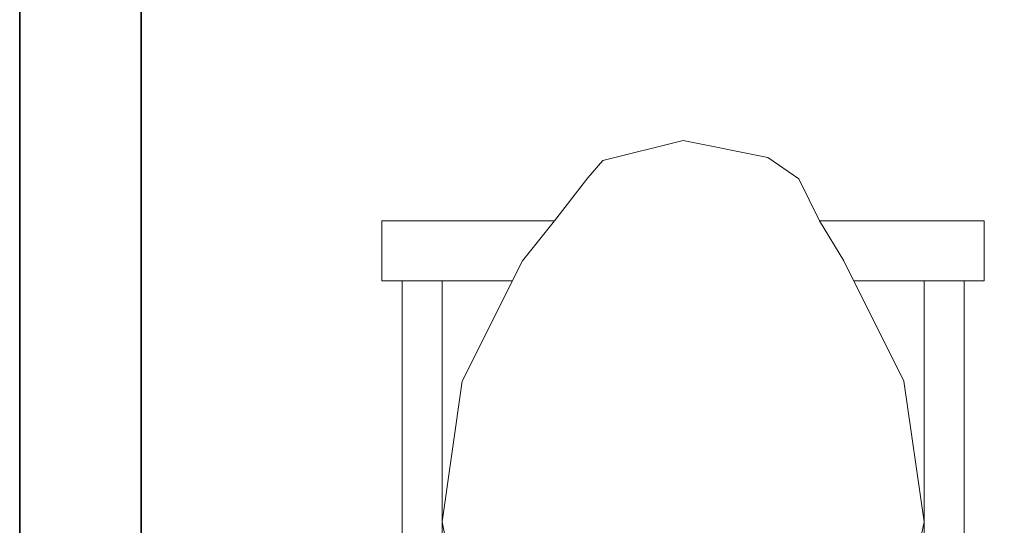
# Model space of a CAD drawing. Units: inches. Extents: x 64 to 1167, y 117 to 939.
# Tile 34 of 56: x 1040 to 1072, y 460 to 476. Entities that reach past the tile are written whole.
import ezdxf

# ---------------------------------------------------------------- set-up
doc = ezdxf.new("R2010")
doc.units = ezdxf.units.IN
doc.header["$MEASUREMENT"] = 0
doc.layers.add('A-FLOR-FIXT', color=8, linetype='Continuous', lineweight=18)
doc.layers.add('A-SECT', color=7, linetype='Continuous', lineweight=35)

# ---------------------------------------------------------------- blocks, each defined once
blk = doc.blocks.new('A$C02040E19')
for p, q in [((201.6, 890.4, 10), (268.8, 907.2, 10)), ((268.8, 907.2, 10), (339.63, 893.03, 10)), ((189.02, 876, 10), (201.6, 890.4, 10)), ((339.63, 893.03, 10), (365.72, 875.01, 10)), ((161.28, 840, 10), (189.02, 876, 10)), ((365.72, 875.01, 10), (383.04, 840, 10)), ((16.8, 840, 10), (161.28, 840, 10)), ((16.8, 840, 10), (16.8, 789.6, 10)), ((16.8, 789.6, 10), (16.8, 840, 10)), ((134.4, 806.4, 10), (161.28, 840, 10)), ((383.04, 840, 10), (520.8, 840, 10)), ((383.04, 840, 10), (403.2, 806.4, 10)), ((520.8, 840, 10), (520.8, 789.6, 10)), ((520.8, 840, 10), (520.8, 789.6, 10)), ((84, 705.6, 10), (134.4, 806.4, 10)), ((403.2, 806.4, 10), (453.6, 705.6, 10)), ((33.6, 789.6, 10), (16.8, 789.6, 10)), ((126, 789.6, 10), (33.6, 789.6, 10)), ((33.6, 403.2, 10), (33.6, 789.6, 10)), ((33.6, 403.2, 10), (33.6, 789.6, 10)), ((67.2, 789.6, 10), (67.2, 403.2, 10)), ((504, 789.6, 10), (411.6, 789.6, 10)), ((470.4, 789.6, 10), (470.4, 403.2, 10)), ((504, 789.6, 10), (504, 403.2, 10)), ((504, 789.6, 10), (504, 403.2, 10)), ((520.8, 789.6, 10), (504, 789.6, 10)), ((84, 705.6, 10), (67.2, 588, 10)), ((453.6, 705.6, 10), (470.4, 588, 10)), ((84, 504, 10), (67.2, 588, 10)), ((84, 504, 10), (67.2, 588, 10)), ((470.4, 588, 10), (453.6, 504, 10)), ((470.4, 588, 10), (453.6, 504, 10)), ((134.4, 436.8, 10), (84, 504, 10)), ((134.4, 436.8, 10), (84, 504, 10)), ((453.6, 504, 10), (403.2, 436.8, 10)), ((403.2, 436.8, 10), (453.6, 504, 10)), ((184.8, 420, 10), (134.4, 436.8, 10)), ((134.4, 436.8, 10), (184.8, 420, 10)), ((403.2, 436.8, 10), (352.8, 420, 10)), ((403.2, 436.8, 10), (352.8, 420, 10)), ((117.6, 403.2, 10), (134.4, 420, 10)), ((134.4, 420, 10), (117.6, 403.2, 10)), ((151.2, 420, 10), (134.4, 420, 10)), ((151.2, 420, 10), (134.4, 420, 10)), ((151.2, 420, 10), (168, 420, 10)), ((168, 420, 10), (151.2, 420, 10)), ((201.6, 420, 10), (168, 420, 10)), ((201.6, 420, 10), (168, 420, 10)), ((201.6, 420, 10), (235.2, 420, 10)), ((201.6, 420, 10), (235.2, 420, 10)), ((268.8, 420, 10), (235.2, 420, 10)), ((268.8, 420, 10), (235.2, 420, 10)), ((268.8, 420, 10), (319.2, 420, 10)), ((268.8, 420, 10), (319.2, 420, 10)), ((336, 420, 10), (319.2, 420, 10)), ((336, 420, 10), (319.2, 420, 10)), ((336, 420, 10), (369.6, 420, 10)), ((369.6, 420, 10), (336, 420, 10)), ((386.4, 420, 10), (369.6, 420, 10)), ((386.4, 420, 10), (369.6, 420, 10)), ((386.4, 420, 10), (403.2, 420, 10)), ((403.2, 420, 10), (386.4, 420, 10)), ((403.2, 420, 10), (420, 403.2, 10)), ((420, 403.2, 10), (403.2, 420, 10)), ((0, 403.2, 10), (0, 285.6, 10)), ((0, 403.2, 10), (33.6, 403.2, 10)), ((33.6, 403.2, 10), (504, 403.2, 10)), ((504, 403.2, 10), (537.6, 403.2, 10)), ((537.6, 403.2, 10), (537.6, 285.6, 10)), ((84, 218.4, 10), (0, 285.6, 10)), ((537.6, 285.6, 10), (453.6, 218.4, 10)), ((100.8, 218.4, 10), (84, 218.4, 10)), ((168, 151.2, 10), (100.8, 218.4, 10)), ((100.8, 218.4, 10), (436.8, 218.4, 10)), ((436.8, 218.4, 10), (369.6, 151.2, 10)), ((436.8, 218.4, 10), (453.6, 218.4, 10)), ((151.2, 16.8, 10), (168, 151.2, 10)), ((168, 151.2, 10), (369.6, 151.2, 10)), ((369.6, 151.2, 10), (386.4, 16.8, 10)), ((151.2, 16.8, 10), (117.6, 16.8, 10)), ((117.6, 0, 10), (117.6, 16.8, 10)), ((151.2, 16.8, 10), (386.4, 16.8, 10)), ((386.4, 16.8, 10), (420, 16.8, 10)), ((420, 16.8, 10), (420, 0, 10)), ((117.6, 0, 10), (420, 0, 10))]:
    blk.add_line(p, q)

msp = doc.modelspace()

# ---------------------------------------------------------------- linework, layer by layer
at = {"layer": 'A-SECT'}
for p, q in [((1039.813, 540.679), (1039.813, 436.679)), ((1043.813, 540.679), (1043.813, 436.679))]:
    msp.add_line(p, q, dxfattribs=at)

# ---------------------------------------------------------------- block references
at = {"layer": 'A-FLOR-FIXT', "xscale": 0.0393700787401575, "yscale": 0.0393700787401575, "zscale": 0.0393700787401575}
msp.add_blockref('A$C02040E19', (1051.087, 436.679, -0.394), dxfattribs=at)

doc.saveas('drawing.dxf')
